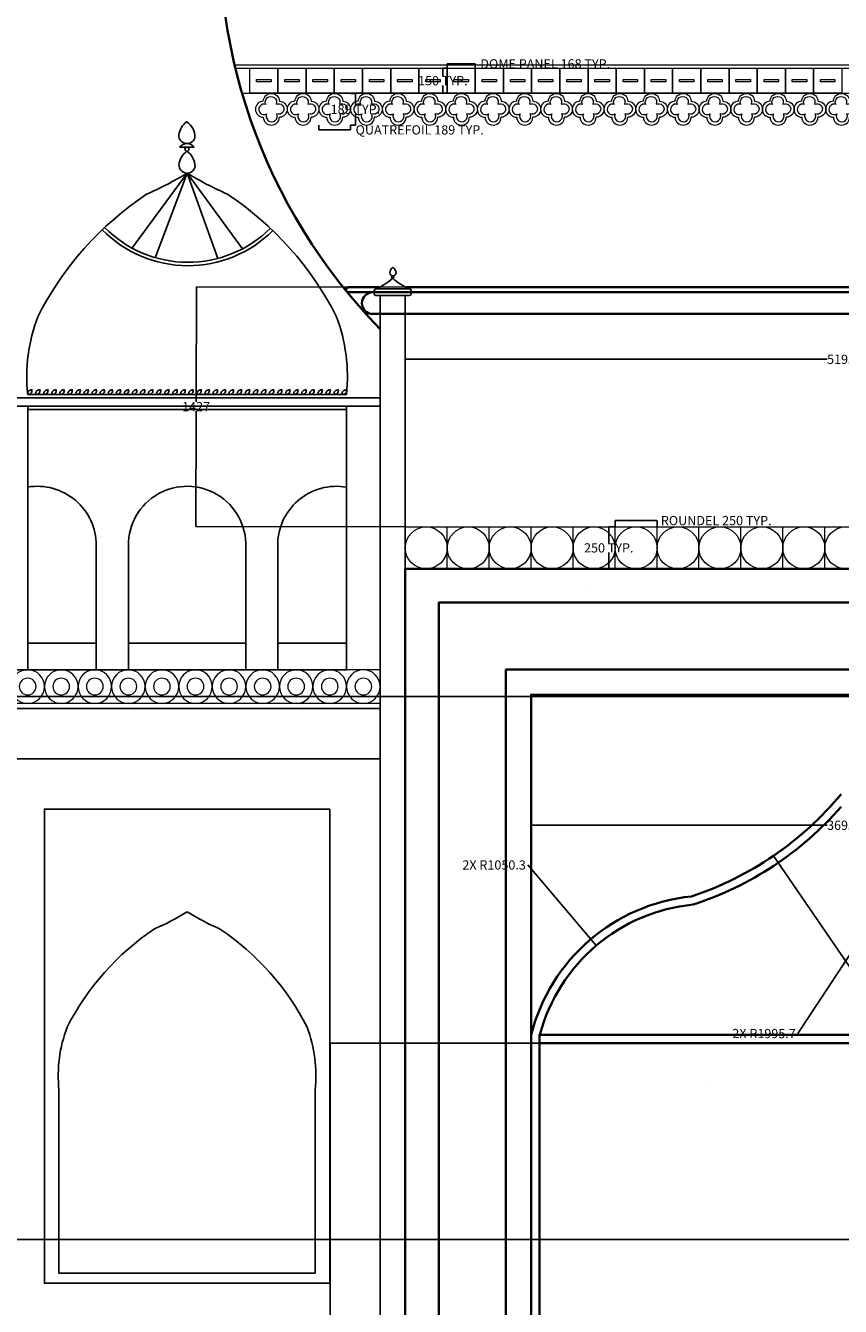
# Model space of a CAD drawing. Units: millimetres. Extents: x 8570 to 49085, y 3782 to 24863.
# Tile 5 of 15: x 17549 to 22404, y 10208 to 17835. Entities that reach past the tile are written whole.
import ezdxf

# ---------------------------------------------------------------- set-up
doc = ezdxf.new("R2010")
doc.units = ezdxf.units.MM
doc.header["$MEASUREMENT"] = 0
doc.header["$PDMODE"] = 3
for name, color, linetype, lineweight in [('A-ANNO-DIMS', 2, 'Continuous', 18), ('A-ELEV', 7, 'Continuous', 25), ('A-ELEV-ARCH', 7, 'Continuous', 25), ('A-ELEV-IWAN', 7, 'Continuous', 35), ('A-ELEV-ORNM', 7, 'Continuous', 13), ('A-ELEV-PIER', 7, 'Continuous', 25), ('A-ROOF-CHAT', 7, 'Continuous', 25), ('A-ROOF-DOME', 7, 'Continuous', 35)]:
    doc.layers.add(name, color=color, linetype=linetype, lineweight=lineweight)
doc.styles.get("Standard").update_dxf_attribs({"font": 'arial.ttf'})
doc.dimstyles.get("Standard").update_dxf_attribs({"dimtxt": 55, "dimasz": 0.18, "dimexe": 0.18, "dimexo": 0.0625, "dimgap": 0.09, "dimtad": 0, "dimtih": 1, "dimtoh": 1, "dimdec": 0, "dimzin": 0, "dimdsep": 46, "dimtxsty": 'Standard', "dimcen": 0.09, "dimadec": 0, "dimazin": 0, "dimtfac": 1, "dimtdec": 0, "dimtofl": 0, "dimtmove": 0, "dimatfit": 3, "dimfxl": 1, "dimtolj": 1, "dimtzin": 0, "dimarcsym": 0})

# ---------------------------------------------------------------- blocks, each defined once
blk = doc.blocks.new('DOME-QUATREFOIL')
for points in [[(46.6, 142.6, -0.970905), (142.6, 142.6, -0.014762)], [(60.6, 123.5, -1.525971), (122.6, 123.9, -0.970905)], [(46.6, 142.6, 0.970905), (46.6, 46.6, 0.014762)], [(63.1, 122.6, 1.61118), (66.6, 66.4, 0.970905)], [(122.6, 123.9, -1.560941), (127.1, 66.6, -0.970905)], [(142.6, 142.6, -0.970905), (142.6, 46.6, -0.014762)], [(46.6, 46.6, 0.970905), (142.6, 46.6, 0.014762)], [(66.6, 66.4, 1.55908), (127.1, 66.6, 0.970905)]]:
    blk.add_lwpolyline(points, format="xyb")
blk = doc.blocks.new('DOME-FRIEZE-PANEL')
for points in [[(0, 150), (168, 150), (168, 0), (0, 0)], [(41, 82), (127, 82), (127, 68), (41, 68)]]:
    blk.add_lwpolyline(points, close=True)
blk = doc.blocks.new('IWAN-EDGE-PINNACLE')
for p, q in [((10, 9044.5), (210, 9044.5)), ((10, 9004.5), (210, 9004.5)), ((35, 0), (35, 9004.5)), ((185, 0), (185, 9004.5))]:
    blk.add_line(p, q)
blk.add_lwpolyline([(127.1, 9142.4, 0.216309), (108.4, 9173.9, 0.244698), (89.5, 9137.5, 0.244698)], format="xyb")
blk.add_circle((110.5, 9116), 7.02)
for centre, radius, start, end in [((-119.7, 9355.4), 336.9, 292.6494, 312.99463), ((108.1, 9141.9), 19, 193.30654, 1.38797), ((340.2, 9356.1), 337.7, 227.0303, 247.32566), ((10, 9034.5), 10, 90, 270), ((10, 9014.5), 10, 90, 270), ((210, 9034.5), 10, 270, 90), ((210, 9014.5), 10, 270, 90)]:
    blk.add_arc(centre, radius, start, end)
blk = doc.blocks.new('ARCADE-RING-FRIEZE')
for p, q in [((0, 200), (2300, 200)), ((2300, 200), (2100, 200)), ((0, 0), (2300, 0))]:
    blk.add_line(p, q)
for centre, radius in [((100, 100), 100), ((300, 100), 100), ((500, 100), 100), ((700, 100), 100), ((900, 100), 100), ((1100, 100), 100), ((1300, 100), 100), ((1500, 100), 100), ((1700, 100), 100), ((1900, 100), 100), ((2100, 100), 100), ((100, 100), 50), ((300, 100), 50), ((500, 100), 50), ((700, 100), 50), ((900, 100), 50), ((1100, 100), 50), ((1300, 100), 50), ((1500, 100), 50), ((1700, 100), 50), ((1900, 100), 50), ((2100, 100), 50)]:
    blk.add_circle(centre, radius)
for radius in [100, 50]:
    blk.add_arc((2300, 100), radius, 90, 270)
blk = doc.blocks.new('CHHATRI-ELEV')
for p, q in [((1107.1, 3111.9), (1194.6, 3111.9)), ((819.3, 2507.3), (1150, 2958.1)), ((967.4, 2449.5), (1150, 2958.1)), ((1480.7, 2507.3), (1150, 2958.1)), ((1339.8, 2454.2), (1150, 2958.1)), ((200, 1639.5), (2100, 1639.5)), ((2300, 1569.5), (2300, 1619.5)), ((200, 1549.5), (2100, 1549.5)), ((610, 0), (610, 754)), ((800, 0), (800, 754)), ((1500, 0), (1500, 744.5)), ((1692, 0), (1692, 744.5)), ((610, 158.5), (200, 158.5)), ((800, 158.5), (1500, 158.5)), ((2100, 158.5), (1692, 158.5))]:
    blk.add_line(p, q)
for points in [[(1199.3, 3183.7, 0.216309), (1151.6, 3264, 0.244698), (1103.6, 3171.4, 0.244698)], [(1198.5, 3007.8, 0.216309), (1150.8, 3088.1, 0.244698), (1102.8, 2995.4, 0.244698)], [(259.6, 2102.5, -0.128405), (908.9, 2832.4, 0.03556), (1150, 2958.1)], [(2040.4, 2102.5, 0.128405), (1391.1, 2832.4, -0.03556), (1150, 2958.1)]]:
    blk.add_lwpolyline(points, format="xyb")
for points in [[(200, 1569.5), (0, 1569.5), (0, 1619.5), (2300, 1619.5), (2300, 1569.5), (2100, 1569.5)], [(2100, 0), (200, 0), (200, 1569.5), (2100, 1569.5), (2100, 0)]]:
    blk.add_lwpolyline(points)
for points in [[(225.8, 1639.5, 0.520567), (200.9, 1667.5, 0.520567)], [(273.9, 1639.5, 0.520567), (249, 1667.5, 0.520567)], [(321.9, 1639.5, 0.520567), (297.1, 1667.5, 0.520567)], [(370, 1639.5, 0.520567), (345.1, 1667.5, 0.520567)], [(418, 1639.5, 0.520567), (393.2, 1667.5, 0.520567)], [(466.1, 1639.5, 0.520567), (441.2, 1667.5, 0.520567)], [(514.2, 1639.5, 0.520567), (489.3, 1667.5, 0.520567)], [(562.2, 1639.5, 0.520567), (537.3, 1667.5, 0.520567)], [(610.3, 1639.5, 0.520567), (585.4, 1667.5, 0.520567)], [(658.3, 1639.5, 0.520567), (633.4, 1667.5, 0.520567)], [(706.4, 1639.5, 0.520567), (681.5, 1667.5, 0.520567)], [(754.4, 1639.5, 0.520567), (729.6, 1667.5, 0.520567)], [(802.5, 1639.5, 0.520567), (777.6, 1667.5, 0.520567)], [(850.5, 1639.5, 0.520567), (825.7, 1667.5, 0.520567)], [(898.6, 1639.5, 0.520567), (873.7, 1667.5, 0.520567)], [(946.7, 1639.5, 0.520567), (921.8, 1667.5, 0.520567)], [(994.7, 1639.5, 0.520567), (969.8, 1667.5, 0.520567)], [(1042.8, 1639.5, 0.520567), (1017.9, 1667.5, 0.520567)], [(1090.8, 1639.5, 0.520567), (1065.9, 1667.5, 0.520567)], [(1138.9, 1639.5, 0.520567), (1114, 1667.5, 0.520567)], [(1186.9, 1639.5, 0.520567), (1162.1, 1667.5, 0.520567)], [(1235, 1639.5, 0.520567), (1210.1, 1667.5, 0.520567)], [(1283, 1639.5, 0.520567), (1258.2, 1667.5, 0.520567)], [(1331.1, 1639.5, 0.520567), (1306.2, 1667.5, 0.520567)], [(1379.2, 1639.5, 0.520567), (1354.3, 1667.5, 0.520567)], [(1427.2, 1639.5, 0.520567), (1402.3, 1667.5, 0.520567)], [(1475.3, 1639.5, 0.520567), (1450.4, 1667.5, 0.520567)], [(1523.3, 1639.5, 0.520567), (1498.4, 1667.5, 0.520567)], [(1571.4, 1639.5, 0.520567), (1546.5, 1667.5, 0.520567)], [(1619.4, 1639.5, 0.520567), (1594.6, 1667.5, 0.520567)], [(1667.5, 1639.5, 0.520567), (1642.6, 1667.5, 0.520567)], [(1715.6, 1639.5, 0.520567), (1690.7, 1667.5, 0.520567)], [(1763.6, 1639.5, 0.520567), (1738.7, 1667.5, 0.520567)], [(1811.7, 1639.5, 0.520567), (1786.8, 1667.5, 0.520567)], [(1859.7, 1639.5, 0.520567), (1834.8, 1667.5, 0.520567)], [(1907.8, 1639.5, 0.520567), (1882.9, 1667.5, 0.520567)], [(1955.8, 1639.5, 0.520567), (1931, 1667.5, 0.520567)], [(2003.9, 1639.5, 0.520567), (1979, 1667.5, 0.520567)], [(2051.9, 1639.5, 0.520567), (2027.1, 1667.5, 0.520567)], [(2100, 1639.5, 0.520567), (2075.1, 1667.5, 0.520567)]]:
    blk.add_lwpolyline(points, format="xyb", close=True)
blk.add_circle((1150.8, 3100), 11.9)
for centre, radius, start, end in [((1150.8, 3182.5), 48.5, 193.30654, 1.38797), ((1150.8, 3079.7), 54.3, 36.37477, 143.62523), ((1150, 3006.6), 48.5, 193.30654, 1.38797), ((1145, 3123.8), 717.3, 225.15569, 315.39684), ((1145, 3123.8), 697.3, 225.15569, 315.39684), ((1217.2, 1743.8), 1022.5, 159.46554, 185.85431), ((1082.8, 1743.8), 1022.5, 354.14569, 20.53446), ((260.1, 742.6), 350.1, 358.13323, 99.88317), ((1149.9, 742.6), 350.1, 359.68831, 181.86677), ((2042.1, 742.6), 350.1, 80.47888, 180.31169)]:
    blk.add_arc(centre, radius, start, end)
blk = doc.blocks.new('WING-UPPER-ARCH')
for p, q in [((86.6, 60), (86.6, 1151.7)), ((1613.4, 60), (1613.4, 1151.7)), ((86.6, 60), (1613.4, 60))]:
    blk.add_line(p, q)
blk.add_lwpolyline([(0, 0), (0, 2823.2), (1700, 2823.2), (1700, 0)], close=True)
for points in [[(134.5, 1523.8, -0.128405), (656.2, 2110.4, 0.03556), (850, 2211.4)], [(1565.5, 1523.8, 0.128405), (1043.8, 2110.4, -0.03556), (850, 2211.4)]]:
    blk.add_lwpolyline(points, format="xyb")
for centre, start, end in [((904, 1235.6), 159.46554, 185.85431), ((796, 1235.6), 354.14569, 20.53446)]:
    blk.add_arc(centre, 821.7, start, end)
blk = doc.blocks.new('IWAN-FRIEZE-ROUNDEL')
blk.add_lwpolyline([(250, 0), (250, 250)])
blk.add_circle((125, 125), 125)
blk = doc.blocks.new('*D37')
at = {"layer": 'A-ANNO-DIMS', "color": 0, "lineweight": -2, "transparency": 16777216}
for p, q in [((20060, 17582.5), (20060, 17607.8)), ((20060.2, 17607.6), (20227.8, 17607.6)), ((20228, 17582.5), (20228, 17607.8)), ((20228, 17607.6), (20228.2, 17607.6))]:
    blk.add_line(p, q, dxfattribs=at)
at = {"layer": 'A-ANNO-DIMS', "color": 0, "transparency": 16777216}
for points in [[(20060.2, 17607.6), (20060.2, 17607.6), (20060, 17607.6)], [(20227.8, 17607.6), (20227.8, 17607.6), (20228, 17607.6)]]:
    blk.add_solid(points, dxfattribs=at)
at = {"layer": 'Defpoints', "color": 0, "transparency": 16777216}
for p in [(20060, 17582.4), (20228, 17607.6), (20228, 17582.4)]:
    blk.add_point(p, dxfattribs=at)
at = {"layer": 'A-ANNO-DIMS', "color": 0, "transparency": 16777216, "insert": (20644.7, 17607.6), "char_height": 55, "attachment_point": 5}
blk.add_mtext('\\A1;DOME PANEL 168 TYP.', dxfattribs=at)
blk = doc.blocks.new('*D38')
at = {"layer": 'A-ANNO-DIMS', "color": 0, "lineweight": -2, "transparency": 16777216}
for p, q in [((20059.9, 17582.4), (20034.6, 17582.4)), ((20034.8, 17582.2), (20034.8, 17535.6)), ((20034.8, 17432.6), (20034.8, 17479.3)), ((20059.9, 17432.4), (20034.6, 17432.4))]:
    blk.add_line(p, q, dxfattribs=at)
at = {"layer": 'A-ANNO-DIMS', "color": 0, "transparency": 16777216}
for points in [[(20034.8, 17582.2), (20034.8, 17582.2), (20034.8, 17582.4)], [(20034.8, 17432.6), (20034.8, 17432.6), (20034.8, 17432.4)]]:
    blk.add_solid(points, dxfattribs=at)
at = {"layer": 'Defpoints', "color": 0, "transparency": 16777216}
for p in [(20034.8, 17582.4), (20060, 17582.4), (20060, 17432.4)]:
    blk.add_point(p, dxfattribs=at)
at = {"layer": 'A-ANNO-DIMS', "color": 0, "transparency": 16777216, "insert": (20034.8, 17507.4), "char_height": 55, "attachment_point": 5}
blk.add_mtext('\\A1;150 TYP.', dxfattribs=at)
blk = doc.blocks.new('*D39')
at = {"layer": 'A-ANNO-DIMS', "color": 0, "lineweight": -2, "transparency": 16777216}
for p, q in [((19295.9, 17242.6), (19295.9, 17214.1)), ((19485.1, 17242.6), (19485.1, 17214.1)), ((19296, 17214.3), (19484.9, 17214.3)), ((19485.1, 17214.3), (19485.3, 17214.3))]:
    blk.add_line(p, q, dxfattribs=at)
at = {"layer": 'A-ANNO-DIMS', "color": 0, "transparency": 16777216}
for points in [[(19296, 17214.3), (19296, 17214.2), (19295.9, 17214.3)], [(19484.9, 17214.3), (19484.9, 17214.2), (19485.1, 17214.3)]]:
    blk.add_solid(points, dxfattribs=at)
at = {"layer": 'Defpoints', "color": 0, "transparency": 16777216}
for p in [(19295.9, 17242.6), (19485.1, 17242.6), (19485.1, 17214.3)]:
    blk.add_point(p, dxfattribs=at)
at = {"layer": 'A-ANNO-DIMS', "color": 0, "transparency": 16777216, "insert": (19896.7, 17214.3), "char_height": 55, "attachment_point": 5}
blk.add_mtext('\\A1;QUATREFOIL 189 TYP.', dxfattribs=at)
blk = doc.blocks.new('*D40')
at = {"layer": 'A-ANNO-DIMS', "color": 0, "lineweight": -2, "transparency": 16777216}
for p, q in [((19485.1, 17431.8), (19513.6, 17431.8)), ((19513.5, 17431.7), (19513.5, 17365.4)), ((19485.1, 17242.6), (19513.6, 17242.6)), ((19513.5, 17242.8), (19513.5, 17309.1))]:
    blk.add_line(p, q, dxfattribs=at)
at = {"layer": 'A-ANNO-DIMS', "color": 0, "transparency": 16777216}
for points in [[(19513.4, 17431.7), (19513.5, 17431.7), (19513.5, 17431.8)], [(19513.4, 17242.8), (19513.5, 17242.8), (19513.5, 17242.6)]]:
    blk.add_solid(points, dxfattribs=at)
at = {"layer": 'Defpoints', "color": 0, "transparency": 16777216}
for p in [(19485.1, 17431.8), (19513.5, 17431.8), (19485.1, 17242.6)]:
    blk.add_point(p, dxfattribs=at)
at = {"layer": 'A-ANNO-DIMS', "color": 0, "transparency": 16777216, "insert": (19513.5, 17337.2), "char_height": 55, "attachment_point": 5}
blk.add_mtext('\\A1;189 TYP.', dxfattribs=at)
blk = doc.blocks.new('*D41')
at = {"layer": 'A-ANNO-DIMS', "color": 0, "lineweight": -2, "transparency": 16777216}
for p, q in [((21061, 14850.1), (21061, 14887.7)), ((21061.2, 14887.5), (21310.8, 14887.5)), ((21311, 14850.1), (21311, 14887.7)), ((21311, 14887.5), (21311.2, 14887.5))]:
    blk.add_line(p, q, dxfattribs=at)
at = {"layer": 'A-ANNO-DIMS', "color": 0, "transparency": 16777216}
for points in [[(21061.2, 14887.5), (21061.2, 14887.5), (21061, 14887.5)], [(21310.8, 14887.5), (21310.8, 14887.5), (21311, 14887.5)]]:
    blk.add_solid(points, dxfattribs=at)
at = {"layer": 'Defpoints', "color": 0, "transparency": 16777216}
for p in [(21311, 14887.5), (21061, 14850), (21311, 14850)]:
    blk.add_point(p, dxfattribs=at)
at = {"layer": 'A-ANNO-DIMS', "color": 0, "transparency": 16777216, "insert": (21663.6, 14887.5), "char_height": 55, "attachment_point": 5}
blk.add_mtext('\\A1;ROUNDEL 250 TYP.', dxfattribs=at)
blk = doc.blocks.new('*D42')
at = {"layer": 'A-ANNO-DIMS', "color": 0, "lineweight": -2, "transparency": 16777216}
for p, q in [((21060.9, 14850), (21023.3, 14850)), ((21023.5, 14849.8), (21023.5, 14753.2)), ((21023.5, 14600.2), (21023.5, 14696.8)), ((21060.9, 14600), (21023.3, 14600))]:
    blk.add_line(p, q, dxfattribs=at)
at = {"layer": 'A-ANNO-DIMS', "color": 0, "transparency": 16777216}
for points in [[(21023.5, 14849.8), (21023.5, 14849.8), (21023.5, 14850)], [(21023.5, 14600.2), (21023.5, 14600.2), (21023.5, 14600)]]:
    blk.add_solid(points, dxfattribs=at)
at = {"layer": 'Defpoints', "color": 0, "transparency": 16777216}
for p in [(21023.5, 14850), (21061, 14850), (21061, 14600)]:
    blk.add_point(p, dxfattribs=at)
at = {"layer": 'A-ANNO-DIMS', "color": 0, "transparency": 16777216, "insert": (21023.5, 14725), "char_height": 55, "attachment_point": 5}
blk.add_mtext('\\A1;250 TYP.', dxfattribs=at)
blk = doc.blocks.new('*D44')
at = {"layer": 'A-ANNO-DIMS', "color": 0, "lineweight": -2, "transparency": 16777216}
for p, q in [((22399.7, 24863), (8684.3, 24863)), ((8684.5, 24862.8), (8684.5, 15410.4)), ((8684.5, 5901.7), (8684.5, 15354.1)), ((10843.9, 5901.5), (8684.3, 5901.5))]:
    blk.add_line(p, q, dxfattribs=at)
at = {"layer": 'A-ANNO-DIMS', "color": 0, "transparency": 16777216}
for points in [[(8684.5, 24862.8), (8684.5, 24862.8), (8684.5, 24863)], [(8684.5, 5901.7), (8684.5, 5901.7), (8684.5, 5901.5)]]:
    blk.add_solid(points, dxfattribs=at)
at = {"layer": 'Defpoints', "color": 0, "transparency": 16777216}
for p in [(8684.5, 24863), (22399.8, 24863), (10844, 5901.5)]:
    blk.add_point(p, dxfattribs=at)
at = {"layer": 'A-ANNO-DIMS', "color": 0, "transparency": 16777216, "insert": (8684.5, 15382.2), "char_height": 55, "attachment_point": 5}
blk.add_mtext('\\A1;18961', dxfattribs=at)
blk = doc.blocks.new('*D47')
at = {"layer": 'A-ANNO-DIMS', "color": 0, "lineweight": -2, "transparency": 16777216}
for p, q in [((19811, 14600.1), (19811, 15848.2)), ((19811.2, 15848), (22325.3, 15848)), ((25003.8, 15848), (22489.7, 15848)), ((25004, 14600.1), (25004, 15848.2))]:
    blk.add_line(p, q, dxfattribs=at)
at = {"layer": 'A-ANNO-DIMS', "color": 0, "transparency": 16777216}
for points in [[(19811.2, 15848), (19811.2, 15848), (19811, 15848)], [(25003.8, 15848), (25003.8, 15848), (25004, 15848)]]:
    blk.add_solid(points, dxfattribs=at)
at = {"layer": 'Defpoints', "color": 0, "transparency": 16777216}
for p in [(25004, 15848), (19811, 14600), (25004, 14600)]:
    blk.add_point(p, dxfattribs=at)
at = {"layer": 'A-ANNO-DIMS', "color": 0, "transparency": 16777216, "insert": (22407.5, 15848), "char_height": 55, "attachment_point": 5}
blk.add_mtext('\\A1;5193', dxfattribs=at)
blk = doc.blocks.new('*D48')
at = {"layer": 'A-ANNO-DIMS', "color": 0, "lineweight": -2, "transparency": 16777216}
for p, q in [((20561, 11825.1), (20561, 13073.2)), ((20561.2, 13073), (22325.3, 13073)), ((24253.8, 13073), (22489.7, 13073)), ((24254, 11825.1), (24254, 13073.2))]:
    blk.add_line(p, q, dxfattribs=at)
at = {"layer": 'A-ANNO-DIMS', "color": 0, "transparency": 16777216}
for points in [[(20561.2, 13073), (20561.2, 13073), (20561, 13073)], [(24253.8, 13073), (24253.8, 13073), (24254, 13073)]]:
    blk.add_solid(points, dxfattribs=at)
at = {"layer": 'Defpoints', "color": 0, "transparency": 16777216}
for p in [(24254, 13073), (20561, 11825), (24254, 11825)]:
    blk.add_point(p, dxfattribs=at)
at = {"layer": 'A-ANNO-DIMS', "color": 0, "transparency": 16777216, "insert": (22407.5, 13073), "char_height": 55, "attachment_point": 5}
blk.add_mtext('\\A1;3693', dxfattribs=at)
blk = doc.blocks.new('*D49')
at = {"layer": 'A-ANNO-DIMS', "color": 0, "lineweight": -2, "transparency": 16777216}
for p, q in [((20610.9, 11775), (19362.8, 11775)), ((19363, 11774.8), (19363, 9526.9)), ((19363, 7222.7), (19363, 9470.6)), ((20610.9, 7222.5), (19362.8, 7222.5))]:
    blk.add_line(p, q, dxfattribs=at)
at = {"layer": 'A-ANNO-DIMS', "color": 0, "transparency": 16777216}
for points in [[(19363, 11774.8), (19363, 11774.8), (19363, 11775)], [(19363, 7222.7), (19363, 7222.7), (19363, 7222.5)]]:
    blk.add_solid(points, dxfattribs=at)
at = {"layer": 'Defpoints', "color": 0, "transparency": 16777216}
for p in [(19363, 11775), (20611, 11775), (20611, 7222.5)]:
    blk.add_point(p, dxfattribs=at)
at = {"layer": 'A-ANNO-DIMS', "color": 0, "transparency": 16777216, "insert": (19363, 9498.7), "char_height": 55, "attachment_point": 5}
blk.add_mtext('\\A1;4552.5', dxfattribs=at)
blk = doc.blocks.new('*D52')
at = {"layer": 'A-ANNO-DIMS', "color": 0, "lineweight": -2, "transparency": 16777216}
for p, q in [((18566.2, 16279.7), (18564.7, 15594)), ((19814.2, 16277), (18566.1, 16279.8)), ((18563, 14853), (18564.6, 15538.6)), ((19810.9, 14850), (18562.8, 14852.8))]:
    blk.add_line(p, q, dxfattribs=at)
at = {"layer": 'A-ANNO-DIMS', "color": 0, "transparency": 16777216}
for points in [[(18566.2, 16279.7), (18566.3, 16279.7), (18566.2, 16279.8)], [(18563, 14853), (18563, 14853), (18563, 14852.8)]]:
    blk.add_solid(points, dxfattribs=at)
at = {"layer": 'Defpoints', "color": 0, "transparency": 16777216}
for p in [(18566.2, 16279.8), (19814.2, 16277), (19811, 14850)]:
    blk.add_point(p, dxfattribs=at)
at = {"layer": 'A-ANNO-DIMS', "color": 0, "transparency": 16777216, "insert": (18564.6, 15566.3), "char_height": 55, "attachment_point": 5}
blk.add_mtext('\\A1;1427', dxfattribs=at)
blk = doc.blocks.new('*D59')
at = {"layer": 'A-ANNO-DIMS', "color": 0, "lineweight": -2, "transparency": 16777216}
for p, q in [((32990.4, 10606.5), (8684.3, 10606.5)), ((8684.5, 10606.3), (8684.5, 8942.7)), ((8684.5, 7222.7), (8684.5, 8886.3)), ((32870.9, 7222.5), (8684.3, 7222.5))]:
    blk.add_line(p, q, dxfattribs=at)
at = {"layer": 'A-ANNO-DIMS', "color": 0, "transparency": 16777216}
for points in [[(8684.5, 10606.3), (8684.5, 10606.3), (8684.5, 10606.5)], [(8684.5, 7222.7), (8684.5, 7222.7), (8684.5, 7222.5)]]:
    blk.add_solid(points, dxfattribs=at)
at = {"layer": 'Defpoints', "color": 0, "transparency": 16777216}
for p in [(8684.5, 10606.5), (32990.5, 10606.5), (32871, 7222.5)]:
    blk.add_point(p, dxfattribs=at)
at = {"layer": 'A-ANNO-DIMS', "color": 0, "transparency": 16777216, "insert": (8684.5, 8914.5), "char_height": 55, "attachment_point": 5}
blk.add_mtext('\\A1;3384', dxfattribs=at)
blk = doc.blocks.new('*D60')
at = {"layer": 'A-ANNO-DIMS', "color": 0, "lineweight": -2, "transparency": 16777216}
for p, q in [((33041.4, 13840.5), (8684.3, 13840.5)), ((8684.5, 13840.3), (8684.5, 12251.7)), ((8684.5, 10606.7), (8684.5, 12195.3)), ((32990.4, 10606.5), (8684.3, 10606.5))]:
    blk.add_line(p, q, dxfattribs=at)
at = {"layer": 'A-ANNO-DIMS', "color": 0, "transparency": 16777216}
for points in [[(8684.5, 13840.3), (8684.5, 13840.3), (8684.5, 13840.5)], [(8684.5, 10606.7), (8684.5, 10606.7), (8684.5, 10606.5)]]:
    blk.add_solid(points, dxfattribs=at)
at = {"layer": 'Defpoints', "color": 0, "transparency": 16777216}
for p in [(8684.5, 13840.5), (33041.5, 13840.5), (32990.5, 10606.5)]:
    blk.add_point(p, dxfattribs=at)
at = {"layer": 'A-ANNO-DIMS', "color": 0, "transparency": 16777216, "insert": (8684.5, 12223.5), "char_height": 55, "attachment_point": 5}
blk.add_mtext('\\A1;3234', dxfattribs=at)
blk = doc.blocks.new('*D61')
at = {"layer": 'A-ANNO-DIMS', "color": 0, "lineweight": -2, "transparency": 16777216}
for p, q in [((33091.4, 17974), (8684.3, 17974)), ((8684.5, 17973.8), (8684.5, 15935.4)), ((8684.5, 13840.7), (8684.5, 15879.1)), ((33041.4, 13840.5), (8684.3, 13840.5))]:
    blk.add_line(p, q, dxfattribs=at)
at = {"layer": 'A-ANNO-DIMS', "color": 0, "transparency": 16777216}
for points in [[(8684.5, 17973.8), (8684.5, 17973.8), (8684.5, 17974)], [(8684.5, 13840.7), (8684.5, 13840.7), (8684.5, 13840.5)]]:
    blk.add_solid(points, dxfattribs=at)
at = {"layer": 'Defpoints', "color": 0, "transparency": 16777216}
for p in [(8684.5, 17974), (33091.5, 17974), (33041.5, 13840.5)]:
    blk.add_point(p, dxfattribs=at)
at = {"layer": 'A-ANNO-DIMS', "color": 0, "transparency": 16777216, "insert": (8684.5, 15907.2), "char_height": 55, "attachment_point": 5}
blk.add_mtext('\\A1;4133.5', dxfattribs=at)
blk = doc.blocks.new('*D81')
at = {"layer": 'A-ANNO-DIMS', "color": 0, "lineweight": -2, "transparency": 16777216}
for p, q in [((23908.1, 14497.3), (23908.1, 14497.5)), ((23908.1, 14497.4), (23908.2, 14497.4)), ((22149.1, 11832.6), (22808.6, 12831.7)), ((22148.9, 11832.6), (22149.1, 11832.6))]:
    blk.add_line(p, q, dxfattribs=at)
at = {"layer": 'A-ANNO-DIMS', "color": 0, "transparency": 16777216}
blk.add_solid([(22808.6, 12831.8), (22808.7, 12831.7), (22808.7, 12831.9)], dxfattribs=at)
at = {"layer": 'Defpoints', "color": 0, "transparency": 16777216}
for p in [(23908.1, 14497.4), (22808.7, 12831.9)]:
    blk.add_point(p, dxfattribs=at)
at = {"layer": 'A-ANNO-DIMS', "color": 0, "transparency": 16777216, "insert": (21948.8, 11832.6), "char_height": 55, "attachment_point": 5}
blk.add_mtext('\\A1;2X R1995.7', dxfattribs=at)
blk = doc.blocks.new('*D82')
at = {"layer": 'A-ANNO-DIMS', "color": 0, "lineweight": -2, "transparency": 16777216}
for p, q in [((20906.8, 14497.4), (20906.9, 14497.4)), ((20906.9, 14497.3), (20906.9, 14497.5)), ((22664, 11927.6), (22005.2, 12891.2)), ((22664.2, 11927.6), (22664, 11927.6))]:
    blk.add_line(p, q, dxfattribs=at)
at = {"layer": 'A-ANNO-DIMS', "color": 0, "transparency": 16777216}
blk.add_solid([(22005.2, 12891.2), (22005.1, 12891.1), (22005.1, 12891.3)], dxfattribs=at)
at = {"layer": 'Defpoints', "color": 0, "transparency": 16777216}
for p in [(20906.9, 14497.4), (22005.1, 12891.3)]:
    blk.add_point(p, dxfattribs=at)
at = {"layer": 'A-ANNO-DIMS', "color": 0, "transparency": 16777216, "insert": (22864.3, 11927.6), "char_height": 55, "attachment_point": 5}
blk.add_mtext('\\A1;2X R1945.7', dxfattribs=at)
blk = doc.blocks.new('*D84')
at = {"layer": 'A-ANNO-DIMS', "color": 0, "lineweight": -2, "transparency": 16777216}
for p, q in [((20540.4, 12836.5), (20540.5, 12836.5)), ((20540.5, 12836.5), (20948.1, 12356.1)), ((21627.6, 11555), (21627.8, 11555)), ((21627.7, 11554.9), (21627.7, 11555.1))]:
    blk.add_line(p, q, dxfattribs=at)
at = {"layer": 'A-ANNO-DIMS', "color": 0, "transparency": 16777216}
blk.add_solid([(20948.1, 12356.1), (20948.1, 12356.1), (20948.2, 12356)], dxfattribs=at)
at = {"layer": 'Defpoints', "color": 0, "transparency": 16777216}
for p in [(20948.2, 12356), (21627.7, 11555)]:
    blk.add_point(p, dxfattribs=at)
at = {"layer": 'A-ANNO-DIMS', "color": 0, "transparency": 16777216, "insert": (20340.2, 12836.5), "char_height": 55, "attachment_point": 5}
blk.add_mtext('\\A1;2X R1050.3', dxfattribs=at)

msp = doc.modelspace()

# ---------------------------------------------------------------- linework, layer by layer
at = {"layer": 'A-ELEV'}
for p, q in [((19661, 13769), (17361, 13769)), ((19661, 13469), (17361, 13469))]:
    msp.add_line(p, q, dxfattribs=at)
at = {"layer": 'A-ELEV-IWAN'}
for points in [[(19811, 7222.5), (19811, 14600), (25004, 14600), (25004, 7222.5)], [(20011, 7222.5), (20011, 14400), (24804, 14400), (24804, 7222.5)], [(20411, 7222.5), (20411, 14000), (24404, 14000), (24404, 7222.5)], [(20561, 7222.5), (20561, 13850)], [(20561, 7222.5), (20561, 13850), (24254, 13850), (24254, 7222.5)], [(20611, 7222.5), (20611, 11825)], [(24202.34, 11825), (20611, 11825)], [(24204, 7222.5), (24204, 11775), (20611, 11775)]]:
    msp.add_lwpolyline(points, dxfattribs=at)
for points in [[(20561, 11825, -0.3152594), (21516.4, 12649.7, 0.1414807), (22407.5, 13259)], [(20612.66, 11825, -0.3133456), (21526.79, 12600.48, 0.1345914), (22407.5, 13181.84, 0.1345914)]]:
    msp.add_lwpolyline(points, format="xyb", dxfattribs=at)
at = {"layer": 'A-ELEV-ORNM'}
for p, q in [((18793.79, 17602.41), (26022.36, 17602.82)), ((18798.6, 17582.41), (26017.56, 17582.82)), ((18838.91, 17432.42), (25940.01, 17432.81)), ((19811, 14850), (25004, 14850))]:
    msp.add_line(p, q, dxfattribs=at)
at = {"layer": 'A-ROOF-DOME'}
for p, q in [((19473.5, 16277), (19657.74, 16277)), ((19473.5, 16247), (25341.5, 16247)), ((19814.24, 16277), (25000.76, 16277)), ((19617, 16118), (25207.5, 16118))]:
    msp.add_line(p, q, dxfattribs=at)
for centre, radius, start, end in [((22070.17, 18381.06), 3367.64, 123.754343, 224.324891), ((19473.5, 16262), 15, 90, 270), ((19617, 16182.5), 64.5, 90, 270)]:
    msp.add_arc(centre, radius, start, end, dxfattribs=at)

# ---------------------------------------------------------------- block references
at = {"layer": 'A-ELEV-ARCH', "extrusion": (0, 0, -1), "zscale": -1}
msp.add_blockref('WING-UPPER-ARCH', (-19361, 10345.75), dxfattribs=at)
at = {"layer": 'A-ELEV-ORNM'}
for name, p in [('DOME-FRIEZE-PANEL', (18884, 17432.43)), ('DOME-FRIEZE-PANEL', (19052, 17432.43)), ('DOME-FRIEZE-PANEL', (19220, 17432.43)), ('DOME-FRIEZE-PANEL', (19388, 17432.43)), ('DOME-FRIEZE-PANEL', (19556, 17432.43)), ('DOME-FRIEZE-PANEL', (19724, 17432.43)), ('DOME-FRIEZE-PANEL', (19892, 17432.43)), ('DOME-FRIEZE-PANEL', (20060, 17432.43)), ('DOME-FRIEZE-PANEL', (20228, 17432.43)), ('DOME-FRIEZE-PANEL', (20396, 17432.43)), ('DOME-FRIEZE-PANEL', (20564, 17432.43)), ('DOME-FRIEZE-PANEL', (20732, 17432.43)), ('DOME-FRIEZE-PANEL', (20900, 17432.43)), ('DOME-FRIEZE-PANEL', (21068, 17432.43)), ('DOME-FRIEZE-PANEL', (21236, 17432.43)), ('DOME-FRIEZE-PANEL', (21404, 17432.43)), ('DOME-FRIEZE-PANEL', (21572, 17432.43)), ('DOME-FRIEZE-PANEL', (21740, 17432.43)), ('DOME-FRIEZE-PANEL', (21908, 17432.43)), ('DOME-FRIEZE-PANEL', (22076, 17432.43)), ('DOME-FRIEZE-PANEL', (22244.01, 17432.43)), ('DOME-QUATREFOIL', (18918.4, 17242.64)), ('DOME-QUATREFOIL', (19107.13, 17242.64)), ('DOME-QUATREFOIL', (19295.87, 17242.64)), ('DOME-QUATREFOIL', (19484.6, 17242.64)), ('DOME-QUATREFOIL', (19673.33, 17242.64)), ('DOME-QUATREFOIL', (19862.06, 17242.64)), ('DOME-QUATREFOIL', (20050.8, 17242.64)), ('DOME-QUATREFOIL', (20239.53, 17242.64)), ('DOME-QUATREFOIL', (20428.26, 17242.64)), ('DOME-QUATREFOIL', (20617, 17242.64)), ('DOME-QUATREFOIL', (20805.73, 17242.64)), ('DOME-QUATREFOIL', (20994.46, 17242.64)), ('DOME-QUATREFOIL', (21183.2, 17242.64)), ('DOME-QUATREFOIL', (21371.93, 17242.64)), ('DOME-QUATREFOIL', (21560.66, 17242.64)), ('DOME-QUATREFOIL', (21749.39, 17242.64)), ('DOME-QUATREFOIL', (21938.13, 17242.64)), ('DOME-QUATREFOIL', (22126.86, 17242.64)), ('DOME-QUATREFOIL', (22315.59, 17242.64)), ('IWAN-FRIEZE-ROUNDEL', (19811, 14600)), ('IWAN-FRIEZE-ROUNDEL', (20061, 14600)), ('IWAN-FRIEZE-ROUNDEL', (20311, 14600)), ('IWAN-FRIEZE-ROUNDEL', (20561, 14600)), ('IWAN-FRIEZE-ROUNDEL', (20811, 14600)), ('IWAN-FRIEZE-ROUNDEL', (21061, 14600)), ('IWAN-FRIEZE-ROUNDEL', (21311, 14600)), ('IWAN-FRIEZE-ROUNDEL', (21561, 14600)), ('IWAN-FRIEZE-ROUNDEL', (21811, 14600)), ('IWAN-FRIEZE-ROUNDEL', (22061, 14600)), ('IWAN-FRIEZE-ROUNDEL', (22311, 14600))]:
    msp.add_blockref(name, p, dxfattribs=at)
at = {"layer": 'A-ELEV-ORNM', "extrusion": (0, 0, -1), "zscale": -1}
msp.add_blockref('ARCADE-RING-FRIEZE', (-19661, 13799), dxfattribs=at)
at = {"layer": 'A-ELEV-PIER', "extrusion": (0, 0, -1), "zscale": -1}
msp.add_blockref('IWAN-EDGE-PINNACLE', (-19846, 7222.5), dxfattribs=at)
at = {"layer": 'A-ROOF-CHAT', "extrusion": (0, 0, -1), "zscale": -1}
msp.add_blockref('CHHATRI-ELEV', (-19661, 13999), dxfattribs=at)

# ---------------------------------------------------------------- dimensions: what is measured, and where the dimension line sits
at = {"layer": 'A-ANNO-DIMS'}
for base, p1, p2, angle, override, picture, middle in [((8684.5, 24862.95), (10844, 5901.5), (22399.75, 24862.95), 90, {"dimdec": 0, "dimlfac": 1, "dimrnd": 0, "dimzin": 0, "dimdsep": 46, "dimlunit": 2}, '*D44', (8684.5, 15382.23)), ((8684.5, 17974), (33041.5, 13840.5), (33091.5, 17974), 90, {"dimdec": 1, "dimlfac": 1, "dimrnd": 0, "dimzin": 0, "dimdsep": 46, "dimlunit": 2}, '*D61', (8684.5, 15907.25)), ((18566.25, 16279.84), (19811, 14850), (19814.24, 16277), 89.869734, {"dimdec": 0, "dimlfac": 1, "dimrnd": 0, "dimzin": 0, "dimdsep": 46, "dimlunit": 2}, '*D52', (18564.63, 15566.34)), ((8684.5, 13840.5), (32990.5, 10606.5), (33041.5, 13840.5), 90, {"dimdec": 0, "dimlfac": 1, "dimrnd": 0, "dimzin": 0, "dimdsep": 46, "dimlunit": 2}, '*D60', (8684.5, 12223.5)), ((19363, 11775), (20611, 7222.5), (20611, 11775), 90, {"dimdec": 1, "dimlfac": 1, "dimrnd": 0, "dimzin": 0, "dimdsep": 46, "dimlunit": 2}, '*D49', (19363, 9498.75)), ((8684.5, 10606.5), (32871, 7222.5), (32990.5, 10606.5), 90, {"dimdec": 0, "dimlfac": 1, "dimrnd": 0, "dimzin": 0, "dimdsep": 46, "dimlunit": 2}, '*D59', (8684.5, 8914.5))]:
    dim = msp.add_linear_dim(base=base, p1=p1, p2=p2, angle=angle, dimstyle='Standard', override=override, dxfattribs=at)
    dim.commit()
    dim.dimension.update_dxf_attribs({"geometry": picture, "text_midpoint": middle})
for base, p1, p2, text, picture, middle in [((20228, 17607.62), (20060, 17582.42), (20228, 17582.42), 'DOME PANEL <> TYP.', '*D37', (20644.71, 17607.62)), ((19485.07, 17214.26), (19295.87, 17242.64), (19485.07, 17242.64), 'QUATREFOIL <> TYP.', '*D39', (19896.66, 17214.26)), ((21311, 14887.5), (21061, 14850), (21311, 14850), 'ROUNDEL <> TYP.', '*D41', (21663.59, 14887.5))]:
    dim = msp.add_linear_dim(base=base, p1=p1, p2=p2, text=text, dimstyle='Standard', override={"dimdec": 0, "dimlfac": 1, "dimrnd": 0, "dimzin": 0, "dimdsep": 46, "dimlunit": 2}, dxfattribs=at)
    dim.commit()
    dim.dimension.update_dxf_attribs({"geometry": picture, "text_midpoint": middle})
for base, p1, p2, picture, middle in [((20034.8, 17582.42), (20060, 17432.43), (20060, 17582.42), '*D38', (20034.8, 17507.42)), ((19513.45, 17431.85), (19485.07, 17242.64), (19485.07, 17431.85), '*D40', (19513.45, 17337.24)), ((21023.5, 14850), (21061, 14600), (21061, 14850), '*D42', (21023.5, 14725))]:
    dim = msp.add_linear_dim(base=base, p1=p1, p2=p2, angle=90, text='<> TYP.', dimstyle='Standard', override={"dimdec": 0, "dimlfac": 1, "dimrnd": 0, "dimzin": 0, "dimdsep": 46, "dimlunit": 2}, dxfattribs=at)
    dim.commit()
    dim.dimension.update_dxf_attribs({"geometry": picture, "text_midpoint": middle})
for base, p1, p2, picture, middle in [((25004, 15848), (19811, 14600), (25004, 14600), '*D47', (22407.5, 15848)), ((24254, 13073), (20561, 11825), (24254, 11825), '*D48', (22407.5, 13073))]:
    dim = msp.add_linear_dim(base=base, p1=p1, p2=p2, dimstyle='Standard', override={"dimdec": 0, "dimlfac": 1, "dimrnd": 0, "dimzin": 0, "dimdsep": 46, "dimlunit": 2}, dxfattribs=at)
    dim.commit()
    dim.dimension.update_dxf_attribs({"geometry": picture, "text_midpoint": middle})
for center, mpoint, picture, middle in [((20906.85, 14497.42), (22005.05, 12891.31), '*D82', (22864.29, 11927.65)), ((23908.15, 14497.42), (22808.73, 12831.89), '*D81', (21948.77, 11832.58)), ((21627.69, 11555.02), (20948.23, 12355.96), '*D84', (20340.24, 12836.53))]:
    dim = msp.add_radius_dim(center=center, mpoint=mpoint, text='2X <>', dimstyle='Standard', override={"dimdec": 1, "dimlfac": 1, "dimrnd": 0, "dimzin": 0, "dimdsep": 46, "dimlunit": 2}, dxfattribs=at)
    dim.commit()
    dim.dimension.update_dxf_attribs({"geometry": picture, "text_midpoint": middle, "dimtype": 164})

doc.saveas('drawing.dxf')
